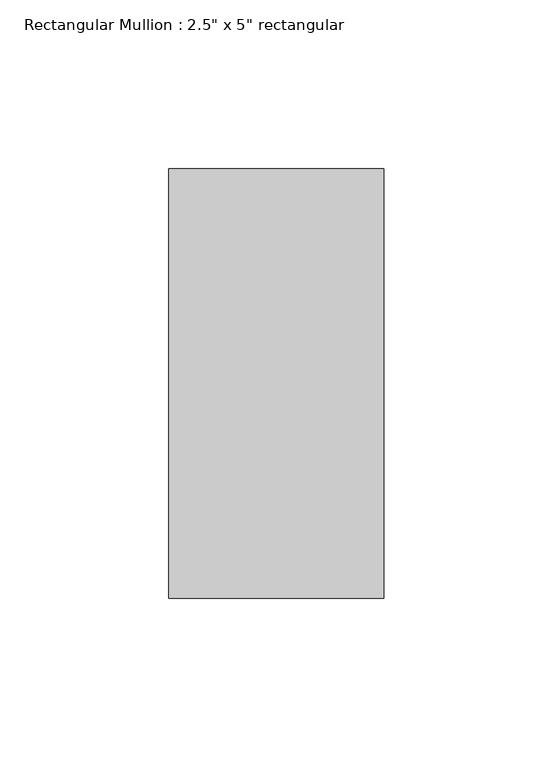
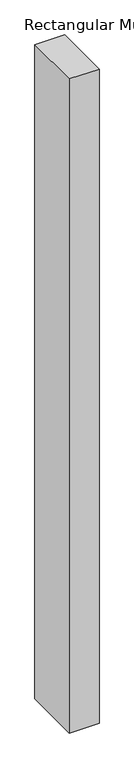
"""IFC4 building model written with IfcOpenShell, lengths in millimetres: member geometry."""

from ifc_helpers import new_model, si_unit, frame, origin, place, context, project, spatial, polyline, outline, extrude, source, transform, mapped, element, save


def member_40abf7f1(model_context):
    return source(origin(), model_context, "Body", "SweptSolid", [
        extrude(outline(polyline([(31.75, 63.5), (31.75, -63.5), (-31.75, -63.5), (-31.75, 63.5), (31.75, 63.5)])), frame((0.0, 0.0, -1475.7821201), z_axis=(0.0, 0.0, 1.0), x_axis=(1.0, 0.0, 0.0)), (0.0, 0.0, 1.0), 1475.7821201),
    ])


if __name__ == "__main__":
    model = new_model("IFC4")
    model_context = context("Model", 3, world=origin())
    ifc_project = project(units=[si_unit("LENGTHUNIT", "METRE", prefix="MILLI")], contexts=[model_context])
    site = spatial("IfcSite", under=ifc_project)
    building = spatial("IfcBuilding", under=site)
    placement = place(None, origin())
    member_shape = member_40abf7f1(model_context)
    element("IfcMember", 1, ObjectType="Rectangular Mullion : 2.5\" x 5\" rectangular", at=placement, inside=building, context=model_context, shape_type="MappedRepresentation", body=[
        mapped(member_shape, transform((0.0, 0.0, 0.0), x_axis=(1.0, 0.0, 0.0), y_axis=(0.0, 1.0, 0.0), z_axis=(0.0, 0.0, 1.0))),
    ])
    save(model, "model.ifc")

# Revit data of these elements
# Type "Rectangular Mullion : 2.5\" x 5\" rectangular"
#   built-in parameter 1007304 = 0.416667 (stored number, unit not read)
#   built-in parameter 1007301 = 0.104167 (stored number, unit not read)
#   built-in parameter 1007300 = 0.104167 (stored number, unit not read)
# Element 1 (IfcMember, "Rectangular Mullion : 2.5\" x 5\" rectangular")
#   Materials on its faces: "Aluminum"
# Materials
#   "Aluminum": class "Metal", colour RGB 247 247 247, transparency 0, Description = "Aluminum 6061", Cost = 0
